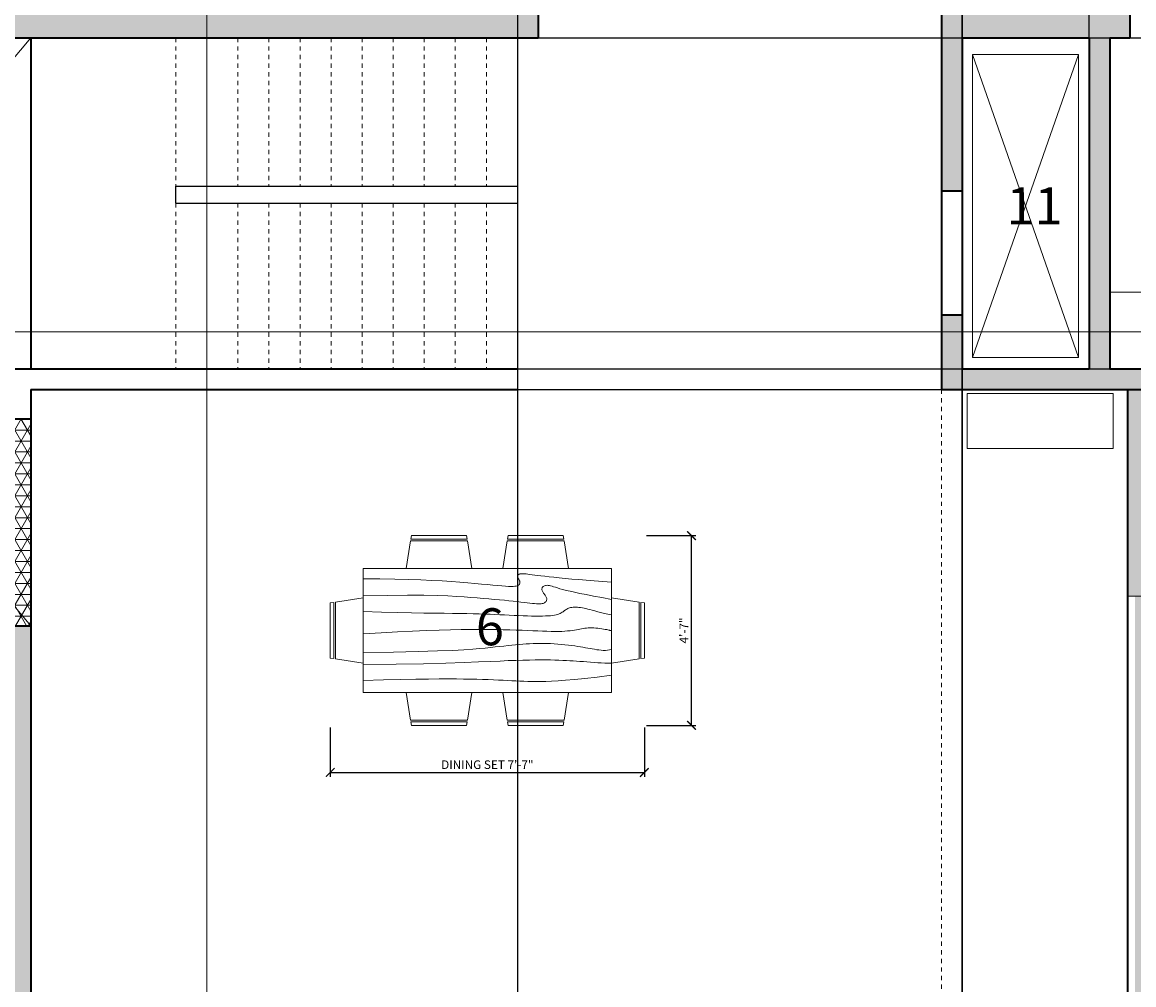
# Model space of a CAD drawing. Units: inches. Extents: x 3122 to 5933, y 1474 to 2995.
# Tile 7 of 12: x 5215 to 5538, y 2360 to 2639. Entities that reach past the tile are written whole.
import ezdxf

# ---------------------------------------------------------------- set-up
doc = ezdxf.new("R2010")
doc.units = ezdxf.units.IN
doc.linetypes.add('JIS_02_1.2', pattern=[2.5, 1.25, -1.25])
for name, color, linetype, lineweight in [('A-ANNO-DIMS', 2, 'Continuous', 18), ('A-ANNO-SYMB', 6, 'Continuous', 18), ('A-AREA-IDEN', 7, 'Continuous', 20), ('A-EQPM', 9, 'Continuous', 20), ('A-FLOR-FIXT', 9, 'Continuous', 18), ('A-FLOR-OPEN', 8, 'Continuous', 13), ('A-FLOR-OVHD', 8, 'JIS_02_1.2', 18), ('A-FLOR-STRS', 7, 'Continuous', 25), ('A-FLOR-STRS-OVHD', 8, 'JIS_02_1.2', 18), ('A-FURN', 8, 'Continuous', 18), ('A-GLAZ', 4, 'Continuous', 18), ('A-WALL', 7, 'Continuous', 35), ('A-WALL-PATT', 7, 'Continuous', 13), ('L-PLNT-PATT', 94, 'Continuous', 13)]:
    doc.layers.add(name, color=color, linetype=linetype, lineweight=lineweight)
doc.styles.get("Standard").update_dxf_attribs({"font": 'arial.ttf'})
doc.dimstyles.new('ISO-25', dxfattribs={"dimtxt": 2.5, "dimasz": 2.5, "dimexe": 1.25, "dimexo": 0.625, "dimtad": 1, "dimdec": 0, "dimlunit": 3, "dimtxsty": 'Standard', "dimblk": 'ARCHTICK', "dimcen": 2.5, "dimadec": 0, "dimazin": 0, "dimtfac": 1, "dimtdec": 0, "dimtmove": 0, "dimatfit": 3, "dimfxl": 1, "dimarcsym": 0})

# ---------------------------------------------------------------- blocks, each defined once
blk = doc.blocks.new('Dining Set - 36 x 72 in.')
for p, q in [((-22.2343, 26.00059), (-23.4847, 17.99762)), ((-22.2304, 26), (-5.7608, 26)), ((-22, 27.5), (-22.1562, 26.50042)), ((-5.8416, 26.5), (-22.1534, 26.5)), ((-22, 27.5), (-6, 27.5)), ((-5.8437, 26.49966), (-6, 27.5)), ((-4.5152, 17.99762), (-5.7655, 25.99926)), ((5.7657, 26.00059), (4.5153, 17.99762)), ((5.7696, 26), (22.2392, 26)), ((6, 27.5), (5.8438, 26.50042)), ((22.1584, 26.5), (5.8466, 26.5)), ((6, 27.5), (22, 27.5)), ((22.1563, 26.49966), (22, 27.5)), ((23.4848, 17.99762), (22.2345, 25.99926)), ((36, 18), (-36, 18)), ((-36, 18), (-36, -18)), ((36, -18), (36, 18)), ((-45.5, 8), (-44.5004, 8.15617)), ((-45.5, 8), (-45.5, -8)), ((-44.5, -8.15843), (-44.5, 8.15338)), ((-44.0006, 8.23428), (-35.9976, 9.48474)), ((-44, 8.23041), (-44, -8.23915)), ((44.0006, 8.23428), (35.9976, 9.48474)), ((44, 8.23041), (44, -8.23915)), ((44.5, -8.15843), (44.5, 8.15338)), ((45.5, 8), (44.5005, 8.15617)), ((45.5, 8), (45.5, -8)), ((-44.4997, -8.15631), (-45.5, -8)), ((-35.9976, -9.48476), (-43.9993, -8.2345)), ((35.9976, -9.48476), (43.9993, -8.2345)), ((44.4997, -8.15631), (45.5, -8)), ((-36, -18), (36, -18)), ((-22.2343, -26.0006), (-23.4847, -17.99762)), ((-4.5152, -17.99762), (-5.7655, -25.99928)), ((5.7657, -26.0006), (4.5153, -17.99762)), ((23.4848, -17.99762), (22.2345, -25.99928)), ((-22.2304, -26), (-5.7608, -26)), ((-22, -27.5), (-22.1562, -26.50044)), ((-5.8416, -26.5), (-22.1534, -26.5)), ((-22, -27.5), (-6, -27.5)), ((-5.8437, -26.49967), (-6, -27.5)), ((5.7696, -26), (22.2392, -26)), ((6, -27.5), (5.8438, -26.50044)), ((22.1584, -26.5), (5.8466, -26.5)), ((6, -27.5), (22, -27.5)), ((22.1563, -26.49967), (22, -27.5))]:
    blk.add_line(p, q)
for points in [[(-36, 15), (-31.1772, 14.97754), (-26.8079, 14.91406), (-22.8538, 14.81543), (-19.276, 14.6875), (-16.0362, 14.53613), (-13.0957, 14.36718), (-10.4159, 14.18652), (-7.9583, 14), (-5.6904, 13.81315), (-3.6035, 13.63021), (-1.6954, 13.45508), (0.0365, 13.29166), (1.5945, 13.14388), (2.9811, 13.01562), (4.1988, 12.9108), (5.25, 12.83333), (6.1393, 12.78613), (6.8802, 12.76823), (7.4883, 12.77767), (7.9792, 12.8125), (8.3685, 12.87077), (8.6719, 12.95052), (8.9049, 13.0498), (9.0833, 13.16666), (9.2205, 13.29899), (9.3216, 13.44401), (9.3895, 13.59879), (9.4271, 13.76041), (9.4373, 13.92594), (9.4232, 14.09245), (9.3875, 14.257), (9.3333, 14.41666), (9.2638, 14.56917), (9.1836, 14.71484), (9.0975, 14.85465), (9.0104, 14.98958), (8.9272, 15.1206), (8.8529, 15.2487), (8.7922, 15.37483), (8.75, 15.5), (8.7305, 15.62467), (8.7344, 15.74739), (8.7617, 15.86621), (8.8125, 15.97916), (8.8867, 16.08431), (8.9844, 16.17968), (9.1055, 16.26334), (9.25, 16.33333), (9.4189, 16.38802), (9.6172, 16.42708), (9.8506, 16.45052), (10.125, 16.45833), (10.4463, 16.45052), (10.8203, 16.42708), (11.2529, 16.38802), (11.75, 16.33333), (12.3184, 16.26318), (12.9694, 16.17838), (13.7151, 16.07991), (14.5677, 15.96875), (15.5395, 15.84586), (16.6426, 15.71224), (17.8893, 15.56884), (19.2917, 15.41666), (20.859, 15.25667), (22.5879, 15.08984), (24.4721, 14.91715), (26.5052, 14.73958), (28.6809, 14.5581), (30.9929, 14.3737), (33.4347, 14.18733), (36, 14)], [(-36, 10), (-28.9766, 10.14274), (-23.1725, 10.20442), (-18.4241, 10.19775), (-14.5677, 10.13541), (-11.4399, 10.03011), (-8.877, 9.89453), (-6.7154, 9.74137), (-4.7917, 9.58333), (-2.9698, 9.43082), (-1.2246, 9.28515), (0.4415, 9.14534), (2.026, 9.01041), (3.5266, 8.87939), (4.9408, 8.7513), (6.266, 8.62516), (7.5, 8.5), (8.6411, 8.37549), (9.6914, 8.2539), (10.6538, 8.13818), (11.5312, 8.03125), (12.3267, 7.93603), (13.043, 7.85547), (13.6831, 7.79248), (14.25, 7.75), (14.7471, 7.7303), (15.1797, 7.73307), (15.5537, 7.75732), (15.875, 7.80208), (16.1494, 7.86637), (16.3828, 7.94922), (16.5811, 8.04964), (16.75, 8.16666), (16.8944, 8.29915), (17.0143, 8.44531), (17.1089, 8.60319), (17.1771, 8.77083), (17.218, 8.94629), (17.2305, 9.1276), (17.2137, 9.31282), (17.1667, 9.5), (17.0895, 9.6875), (16.987, 9.875), (16.8649, 10.0625), (16.7292, 10.25), (16.5856, 10.4375), (16.4401, 10.625), (16.2985, 10.8125), (16.1667, 11), (16.05, 11.18733), (15.9518, 11.3737), (15.8752, 11.5581), (15.8229, 11.73958), (15.798, 11.91715), (15.8034, 12.08984), (15.842, 12.25667), (15.9167, 12.41666), (16.0295, 12.56836), (16.1784, 12.70833), (16.3605, 12.83268), (16.5729, 12.9375), (16.8127, 13.01888), (17.0768, 13.07291), (17.3625, 13.0957), (17.6667, 13.08333), (17.9894, 13.03312), (18.3418, 12.94726), (18.7382, 12.82918), (19.1927, 12.68229), (19.7195, 12.51001), (20.3327, 12.31575), (21.0465, 12.10294), (21.875, 11.875), (22.8357, 11.63354), (23.959, 11.37304), (25.2786, 11.08618), (26.8282, 10.76562), (28.6414, 10.40405), (30.752, 9.99414), (33.1936, 9.52856), (36, 9)], [(-36, 5.5), (-30.7157, 5.3348), (-26.069, 5.20963), (-21.9946, 5.11767), (-18.4271, 5.05208), (-15.3009, 5.00602), (-12.5508, 4.97265), (-10.1112, 4.94515), (-7.9167, 4.91666), (-5.909, 4.88167), (-4.0586, 4.83984), (-2.3429, 4.79215), (-0.7396, 4.73958), (0.7739, 4.6831), (2.22, 4.6237), (3.6213, 4.56233), (5, 4.5), (6.373, 4.43782), (7.7344, 4.3776), (9.0723, 4.32129), (10.375, 4.27083), (11.6309, 4.22819), (12.8281, 4.19531), (13.9551, 4.17415), (15, 4.16666), (15.954, 4.17448), (16.819, 4.19791), (17.6001, 4.23698), (18.3021, 4.29166), (18.9299, 4.36198), (19.4883, 4.44791), (19.9823, 4.54948), (20.4167, 4.66666), (20.7969, 4.79899), (21.1302, 4.94401), (21.4245, 5.09879), (21.6875, 5.26041), (21.9271, 5.42594), (22.1511, 5.59245), (22.3672, 5.757), (22.5834, 5.91666), (22.8065, 6.06868), (23.0404, 6.21093), (23.2879, 6.34147), (23.5521, 6.45833), (23.8358, 6.55957), (24.142, 6.64323), (24.4735, 6.70735), (24.8334, 6.75), (25.2235, 6.76969), (25.642, 6.76692), (26.0858, 6.74267), (26.5521, 6.69791), (27.0379, 6.63362), (27.5404, 6.55078), (28.0565, 6.45036), (28.5834, 6.33333), (29.1242, 6.19987), (29.7071, 6.04687), (30.3661, 5.87044), (31.1354, 5.66666), (32.0493, 5.43164), (33.142, 5.16146), (34.4475, 4.85221), (36, 4.5)], [(-36, -1), (-30.7915, -0.6591), (-26.0195, -0.38216), (-21.6519, -0.16284), (-17.6563, 0.00521), (-14.0005, 0.12833), (-10.6523, 0.21289), (-7.5796, 0.26522), (-4.75, 0.29166), (-2.134, 0.29793), (0.2878, 0.28711), (2.5317, 0.26163), (4.6146, 0.22396), (6.5529, 0.17651), (8.3633, 0.12174), (10.0623, 0.06209), (11.6667, 0), (13.1899, -0.06201), (14.6341, -0.1211), (15.9982, -0.17432), (17.2813, -0.21875), (18.4823, -0.25147), (19.6003, -0.26953), (20.6343, -0.27002), (21.5834, -0.25), (22.4481, -0.20768), (23.2357, -0.14584), (23.9549, -0.06836), (24.6146, 0.02083), (25.2235, 0.11784), (25.7904, 0.21875), (26.3241, 0.31966), (26.8334, 0.41666), (27.3265, 0.50618), (27.8099, 0.58593), (28.2894, 0.65397), (28.7709, 0.70833), (29.2601, 0.74707), (29.763, 0.76823), (30.2855, 0.76985), (30.8334, 0.75), (31.4088, 0.70784), (31.9994, 0.64713), (32.589, 0.57275), (33.1615, 0.48958), (33.7008, 0.4025), (34.1908, 0.3164), (34.6153, 0.23616), (34.9584, 0.16666), (35.2099, 0.11165), (35.3848, 0.07031), (35.504, 0.04069), (35.5886, 0.02083), (35.6594, 0.00879), (35.7377, 0.0026), (35.8442, 0.00032), (36, 0)], [(-36, -6.5), (-27.1843, -6.31267), (-20.084, -6.1263), (-14.469, -5.9419), (-10.1094, -5.76042), (-6.7752, -5.58285), (-4.2363, -5.41016), (-2.2629, -5.24333), (-0.625, -5.08334), (0.8708, -4.93099), (2.2715, -4.78646), (3.5872, -4.64974), (4.8281, -4.52084), (6.0046, -4.39974), (7.127, -4.28646), (8.2053, -4.18099), (9.25, -4.08334), (10.2705, -3.99382), (11.2734, -3.91407), (12.2647, -3.84603), (13.25, -3.79167), (14.2354, -3.75293), (15.2266, -3.73177), (16.2295, -3.73015), (17.25, -3.75), (18.2912, -3.79248), (19.3451, -3.85547), (20.4009, -3.93604), (21.4479, -4.03125), (22.4754, -4.13819), (23.4727, -4.25391), (24.4289, -4.37549), (25.3334, -4.5), (26.1785, -4.62492), (26.9694, -4.74935), (27.7145, -4.87281), (28.4219, -4.99479), (29.1, -5.11483), (29.7572, -5.23242), (30.4016, -5.34709), (31.0417, -5.45834), (31.6837, -5.56437), (32.3262, -5.65821), (32.9658, -5.73153), (33.599, -5.77604), (34.2224, -5.78345), (34.8327, -5.74545), (35.4264, -5.65373), (36, -5.5)], [(-36, -10), (-26.4022, -9.81299), (-18.4675, -9.62891), (-11.9839, -9.45069), (-6.7396, -9.28125), (-2.5226, -9.12354), (0.8789, -8.98047), (3.6769, -8.85498), (6.0833, -8.75), (8.2767, -8.66765), (10.3021, -8.60677), (12.1712, -8.56543), (13.8958, -8.54167), (15.4876, -8.53353), (16.9583, -8.53907), (18.3197, -8.55632), (19.5834, -8.58334), (20.7616, -8.61841), (21.8685, -8.66081), (22.9188, -8.71004), (23.9271, -8.76563), (24.9081, -8.82707), (25.8763, -8.89388), (26.8465, -8.96558), (27.8334, -9.04167), (28.8474, -9.12118), (29.8828, -9.20117), (30.93, -9.27824), (31.9792, -9.34896), (33.0205, -9.40991), (34.0443, -9.45768), (35.0407, -9.48885), (36, -9.5)], [(-36, -14.5), (-30.0881, -14.33513), (-25.0332, -14.21224), (-20.7312, -14.12647), (-17.0781, -14.07292), (-13.97, -14.04671), (-11.3027, -14.04297), (-8.9724, -14.05681), (-6.875, -14.08334), (-4.9224, -14.11833), (-3.0905, -14.16016), (-1.3709, -14.20785), (0.2448, -14.26042), (1.7647, -14.3169), (3.1973, -14.3763), (4.5507, -14.43767), (5.8333, -14.5), (7.0554, -14.5621), (8.235, -14.62175), (9.3922, -14.67652), (10.5469, -14.72396), (11.7192, -14.76164), (12.929, -14.78711), (14.1965, -14.79794), (15.5417, -14.79167), (16.9933, -14.76424), (18.6152, -14.70508), (20.4804, -14.60197), (22.6615, -14.44271), (25.2312, -14.21509), (28.2624, -13.9069), (31.8277, -13.50594), (36, -13)]]:
    blk.add_lwpolyline(points)
blk = doc.blocks.new('_ArchTick')
at = {"color": 0, "linetype": 'ByBlock', "const_width": 0.15}
blk.add_lwpolyline([(-0.5, -0.5), (0.5, 0.5)], dxfattribs=at)
blk = doc.blocks.new('*D82')
at = {"layer": 'A-ANNO-DIMS', "color": 0, "lineweight": -2, "transparency": 16777216}
for p, q in [((5304.74, 2434.72), (5304.74, 2420.45)), ((5395.74, 2434.72), (5395.74, 2420.45)), ((5304.74, 2421.7), (5395.74, 2421.7))]:
    blk.add_line(p, q, dxfattribs=at)
at = {"layer": 'Defpoints', "color": 0, "transparency": 16777216}
for p in [(5304.74, 2435.35), (5395.74, 2435.35), (5395.74, 2421.7)]:
    blk.add_point(p, dxfattribs=at)
at = {"layer": 'A-ANNO-DIMS', "color": 0, "lineweight": -2, "transparency": 16777216, "xscale": 2.5, "yscale": 2.5, "zscale": 2.5, "rotation": 180}
blk.add_blockref('_ArchTick', (5304.74, 2421.7), dxfattribs=at)
at = {"layer": 'A-ANNO-DIMS', "color": 0, "lineweight": -2, "transparency": 16777216, "xscale": 2.5, "yscale": 2.5, "zscale": 2.5}
blk.add_blockref('_ArchTick', (5395.74, 2421.7), dxfattribs=at)
at = {"layer": 'A-ANNO-DIMS', "color": 0, "transparency": 16777216, "insert": (5350.24, 2423.62), "char_height": 2.5, "attachment_point": 5}
blk.add_mtext('DINING SET 7\'-7"', dxfattribs=at)
blk = doc.blocks.new('*D83')
at = {"layer": 'A-ANNO-DIMS', "color": 0, "lineweight": -2, "transparency": 16777216}
for p, q in [((5396.36, 2490.35), (5410.64, 2490.35)), ((5409.39, 2435.35), (5409.39, 2490.35)), ((5396.36, 2435.35), (5410.64, 2435.35))]:
    blk.add_line(p, q, dxfattribs=at)
at = {"layer": 'Defpoints', "color": 0, "transparency": 16777216}
for p in [(5395.74, 2490.35), (5409.39, 2490.35), (5395.74, 2435.35)]:
    blk.add_point(p, dxfattribs=at)
at = {"layer": 'A-ANNO-DIMS', "color": 0, "lineweight": -2, "transparency": 16777216, "xscale": 2.5, "yscale": 2.5, "zscale": 2.5}
for p, rotation in [((5409.39, 2490.35), 90), ((5409.39, 2435.35), 270)]:
    blk.add_blockref('_ArchTick', p, dxfattribs=dict(at, rotation=rotation))
at = {"layer": 'A-ANNO-DIMS', "color": 0, "transparency": 16777216, "insert": (5407.51, 2462.85), "char_height": 2.5, "attachment_point": 5, "rotation": 90}
blk.add_mtext('4\'-7"', dxfattribs=at)
blk = doc.blocks.new('*D94')
at = {"layer": 'A-ANNO-DIMS', "color": 0, "lineweight": -2, "transparency": 16777216}
for p, q in [((5064.96, 1916.52), (5064.96, 2990.75)), ((5064.96, 2989.5), (5487.87, 2989.5)), ((5487.87, 1916.52), (5487.87, 2990.75))]:
    blk.add_line(p, q, dxfattribs=at)
at = {"layer": 'Defpoints', "color": 0, "transparency": 16777216}
for p in [(5487.87, 2989.5), (5064.96, 1915.9), (5487.87, 1915.9)]:
    blk.add_point(p, dxfattribs=at)
at = {"layer": 'A-ANNO-DIMS', "color": 0, "lineweight": -2, "transparency": 16777216, "xscale": 2.5, "yscale": 2.5, "zscale": 2.5, "rotation": 180}
blk.add_blockref('_ArchTick', (5064.96, 2989.5), dxfattribs=at)
at = {"layer": 'A-ANNO-DIMS', "color": 0, "lineweight": -2, "transparency": 16777216, "xscale": 2.5, "yscale": 2.5, "zscale": 2.5}
blk.add_blockref('_ArchTick', (5487.87, 2989.5), dxfattribs=at)
at = {"layer": 'A-ANNO-DIMS', "color": 0, "transparency": 16777216, "insert": (5276.42, 2991.41), "char_height": 2.5, "attachment_point": 5}
blk.add_mtext('35\'-3"', dxfattribs=at)
blk = doc.blocks.new('*D108')
at = {"layer": 'A-ANNO-DIMS', "color": 0, "lineweight": -2, "transparency": 16777216}
for p, q in [((5178.96, 2643.06), (5178.96, 1792.93)), ((5358.96, 2643.06), (5358.96, 1792.93)), ((5178.96, 1794.18), (5358.96, 1794.18))]:
    blk.add_line(p, q, dxfattribs=at)
at = {"layer": 'Defpoints', "color": 0, "transparency": 16777216}
for p in [(5178.96, 2643.69), (5358.96, 2643.69), (5358.96, 1794.18)]:
    blk.add_point(p, dxfattribs=at)
at = {"layer": 'A-ANNO-DIMS', "color": 0, "lineweight": -2, "transparency": 16777216, "xscale": 2.5, "yscale": 2.5, "zscale": 2.5, "rotation": 180}
blk.add_blockref('_ArchTick', (5178.96, 1794.18), dxfattribs=at)
at = {"layer": 'A-ANNO-DIMS', "color": 0, "lineweight": -2, "transparency": 16777216, "xscale": 2.5, "yscale": 2.5, "zscale": 2.5}
blk.add_blockref('_ArchTick', (5358.96, 1794.18), dxfattribs=at)
at = {"layer": 'A-ANNO-DIMS', "color": 0, "transparency": 16777216, "insert": (5268.96, 1796.08), "char_height": 2.5, "attachment_point": 5}
blk.add_mtext('15\'-0"', dxfattribs=at)
blk = doc.blocks.new('*D110')
at = {"layer": 'A-ANNO-DIMS', "color": 0, "lineweight": -2, "transparency": 16777216}
for p, q in [((5487.87, 2643.06), (5487.87, 1792.93)), ((5670.96, 2643.06), (5670.96, 1792.93)), ((5487.87, 1794.18), (5670.96, 1794.18))]:
    blk.add_line(p, q, dxfattribs=at)
at = {"layer": 'Defpoints', "color": 0, "transparency": 16777216}
for p in [(5487.87, 2643.69), (5670.96, 2643.69), (5670.96, 1794.18)]:
    blk.add_point(p, dxfattribs=at)
at = {"layer": 'A-ANNO-DIMS', "color": 0, "lineweight": -2, "transparency": 16777216, "xscale": 2.5, "yscale": 2.5, "zscale": 2.5, "rotation": 180}
blk.add_blockref('_ArchTick', (5487.87, 1794.18), dxfattribs=at)
at = {"layer": 'A-ANNO-DIMS', "color": 0, "lineweight": -2, "transparency": 16777216, "xscale": 2.5, "yscale": 2.5, "zscale": 2.5}
blk.add_blockref('_ArchTick', (5670.96, 1794.18), dxfattribs=at)
at = {"layer": 'A-ANNO-DIMS', "color": 0, "transparency": 16777216, "insert": (5579.42, 1796.09), "char_height": 2.5, "attachment_point": 5}
blk.add_mtext('15\'-3"', dxfattribs=at)
blk = doc.blocks.new('*D113')
at = {"layer": 'A-ANNO-DIMS', "color": 0, "lineweight": -2, "transparency": 16777216}
for p, q in [((5218.59, 2634.69), (5931.98, 2634.69)), ((5930.73, 2538.69), (5930.73, 2634.69)), ((5218.59, 2538.69), (5931.98, 2538.69))]:
    blk.add_line(p, q, dxfattribs=at)
at = {"layer": 'Defpoints', "color": 0, "transparency": 16777216}
for p in [(5217.96, 2634.69), (5930.73, 2634.69), (5217.96, 2538.69)]:
    blk.add_point(p, dxfattribs=at)
at = {"layer": 'A-ANNO-DIMS', "color": 0, "lineweight": -2, "transparency": 16777216, "xscale": 2.5, "yscale": 2.5, "zscale": 2.5}
for p, rotation in [((5930.73, 2634.69), 90), ((5930.73, 2538.69), 270)]:
    blk.add_blockref('_ArchTick', p, dxfattribs=dict(at, rotation=rotation))
at = {"layer": 'A-ANNO-DIMS', "color": 0, "transparency": 16777216, "insert": (5928.83, 2586.69), "char_height": 2.5, "attachment_point": 5, "rotation": 90}
blk.add_mtext('8\'-0"', dxfattribs=at)
blk = doc.blocks.new('*D114')
at = {"layer": 'A-ANNO-DIMS', "color": 0, "lineweight": -2, "transparency": 16777216}
for p, q in [((5487.87, 2539.31), (5487.87, 2990.75)), ((5487.87, 2989.5), (5524.65, 2989.5)), ((5524.65, 2539.31), (5524.65, 2990.75))]:
    blk.add_line(p, q, dxfattribs=at)
at = {"layer": 'Defpoints', "color": 0, "transparency": 16777216}
for p in [(5524.65, 2989.5), (5487.87, 2538.69), (5524.65, 2538.69)]:
    blk.add_point(p, dxfattribs=at)
at = {"layer": 'A-ANNO-DIMS', "color": 0, "lineweight": -2, "transparency": 16777216, "xscale": 2.5, "yscale": 2.5, "zscale": 2.5, "rotation": 180}
blk.add_blockref('_ArchTick', (5487.87, 2989.5), dxfattribs=at)
at = {"layer": 'A-ANNO-DIMS', "color": 0, "lineweight": -2, "transparency": 16777216, "xscale": 2.5, "yscale": 2.5, "zscale": 2.5}
blk.add_blockref('_ArchTick', (5524.65, 2989.5), dxfattribs=at)
at = {"layer": 'A-ANNO-DIMS', "color": 0, "transparency": 16777216, "insert": (5506.26, 2991.41), "char_height": 2.5, "attachment_point": 5}
blk.add_mtext('3\'-1"', dxfattribs=at)
blk = doc.blocks.new('*D115')
at = {"layer": 'A-ANNO-DIMS', "color": 0, "lineweight": -2, "transparency": 16777216}
for p, q in [((5217.96, 2532.06), (5217.96, 1792.93)), ((5535.87, 2532.06), (5535.87, 1792.93)), ((5217.96, 1794.18), (5535.87, 1794.18))]:
    blk.add_line(p, q, dxfattribs=at)
at = {"layer": 'Defpoints', "color": 0, "transparency": 16777216}
for p in [(5217.96, 2532.69), (5535.87, 2532.69), (5535.87, 1794.18)]:
    blk.add_point(p, dxfattribs=at)
at = {"layer": 'A-ANNO-DIMS', "color": 0, "lineweight": -2, "transparency": 16777216, "xscale": 2.5, "yscale": 2.5, "zscale": 2.5, "rotation": 180}
blk.add_blockref('_ArchTick', (5217.96, 1794.18), dxfattribs=at)
at = {"layer": 'A-ANNO-DIMS', "color": 0, "lineweight": -2, "transparency": 16777216, "xscale": 2.5, "yscale": 2.5, "zscale": 2.5}
blk.add_blockref('_ArchTick', (5535.87, 1794.18), dxfattribs=at)
at = {"layer": 'A-ANNO-DIMS', "color": 0, "transparency": 16777216, "insert": (5376.92, 1796.08), "char_height": 2.5, "attachment_point": 5}
blk.add_mtext('26\'-6"', dxfattribs=at)
blk = doc.blocks.new('*D116')
at = {"layer": 'A-ANNO-DIMS', "color": 0, "lineweight": -2, "transparency": 16777216}
for p, q in [((5218.59, 2532.69), (5931.98, 2532.69)), ((5930.73, 2352.69), (5930.73, 2532.69)), ((5218.59, 2352.69), (5931.98, 2352.69))]:
    blk.add_line(p, q, dxfattribs=at)
at = {"layer": 'Defpoints', "color": 0, "transparency": 16777216}
for p in [(5217.96, 2532.69), (5930.73, 2532.69), (5217.96, 2352.69)]:
    blk.add_point(p, dxfattribs=at)
at = {"layer": 'A-ANNO-DIMS', "color": 0, "lineweight": -2, "transparency": 16777216, "xscale": 2.5, "yscale": 2.5, "zscale": 2.5}
for p, rotation in [((5930.73, 2532.69), 90), ((5930.73, 2352.69), 270)]:
    blk.add_blockref('_ArchTick', p, dxfattribs=dict(at, rotation=rotation))
at = {"layer": 'A-ANNO-DIMS', "color": 0, "transparency": 16777216, "insert": (5928.83, 2442.69), "char_height": 2.5, "attachment_point": 5, "rotation": 90}
blk.add_mtext('15\'-0"', dxfattribs=at)

msp = doc.modelspace()

# ---------------------------------------------------------------- hatches: boundary and pattern name
at = {"layer": 'A-WALL-PATT'}
h = msp.add_hatch(color=256, dxfattribs=at)
h.dxf.hatch_style = 1
h.paths.add_polyline_path([(5073.96, 2454.69), (5101.59, 2454.69), (5101.59, 2459.69), (5101.59, 2463.69), (5073.96, 2463.69), (5073.96, 2634.69), (5169.96, 2634.69), (5364.96, 2634.69), (5364.96, 2643.69), (5364.96, 2667.06), (5358.96, 2667.06), (5358.96, 2643.69), (5178.96, 2643.69), (5178.96, 2655.69), (5169.96, 2655.69), (5169.96, 2643.69), (5073.96, 2643.69), (5073.96, 2745.9), (5124.13, 2745.9), (5124.13, 2754.9), (5073.96, 2754.9), (5073.96, 2866.9), (5169.96, 2866.9), (5169.96, 2818.9), (5169.96, 2812.9), (5169.96, 2754.9), (5154.13, 2754.9), (5154.13, 2745.9), (5169.96, 2745.9), (5169.96, 2691.69), (5178.96, 2691.69), (5178.96, 2812.9), (5178.96, 2818.9), (5178.96, 2875.9), (5064.96, 2875.9), (5064.96, 2055.71), (5217.96, 2055.71), (5217.96, 2464.19), (5212.96, 2464.19), (5212.96, 2463.69), (5148.19, 2463.69), (5148.19, 2459.69), (5148.19, 2454.69), (5158.96, 2454.69), (5158.96, 2450.72), (5156.04, 2450.72), (5156.04, 2447.72), (5158.96, 2447.72), (5158.96, 2425.1), (5164.96, 2425.1), (5164.96, 2447.72), (5167.71, 2447.72), (5167.71, 2450.72), (5164.96, 2450.72), (5164.96, 2454.69), (5212.96, 2454.69), (5212.96, 2064.71), (5073.96, 2064.71), (5073.96, 2322.69), (5158.96, 2322.69), (5164.96, 2322.69), (5164.96, 2328.69), (5158.96, 2328.69), (5073.96, 2328.69)])
h = msp.add_hatch(color=256, dxfattribs=at)
h.dxf.hatch_style = 1
h.paths.add_polyline_path([(5536.42, 2643.69), (5487.87, 2643.69), (5487.87, 2667.06), (5485.81, 2667.06), (5481.87, 2667.06), (5481.87, 2643.69), (5481.87, 2590.35), (5487.87, 2590.35), (5487.87, 2634.69), (5524.65, 2634.69), (5524.65, 2538.69), (5487.87, 2538.69), (5487.87, 2554.35), (5481.87, 2554.35), (5481.87, 2532.69), (5524.65, 2532.69), (5658.65, 2532.69), (5718.65, 2532.69), (5718.65, 2501.93), (5724.65, 2501.93), (5724.65, 2549.4), (5718.65, 2549.4), (5718.65, 2538.69), (5658.65, 2538.69), (5658.65, 2573.57), (5658.59, 2573.63), (5654.65, 2573.63), (5654.65, 2538.69), (5594.65, 2538.69), (5594.65, 2573.57), (5594.59, 2573.63), (5590.65, 2573.63), (5590.65, 2538.69), (5530.65, 2538.69), (5530.65, 2634.69), (5536.42, 2634.69)])
h.paths.add_polyline_path([(5735.69, 2643.69), (5679.96, 2643.69), (5679.96, 2710.77), (5720.44, 2710.77), (5720.44, 2687.32), (5737.79, 2687.32), (5737.79, 2692.32), (5725.44, 2692.32), (5725.44, 2715.77), (5679.96, 2715.77), (5679.96, 2866.9), (5775.96, 2866.9), (5775.96, 2692.32), (5773.79, 2692.32), (5773.79, 2687.32), (5775.96, 2687.32), (5775.96, 2643.69), (5775.96, 2591.85), (5784.96, 2591.85), (5784.96, 2875.9), (5670.96, 2875.9), (5670.96, 2818.9), (5412.4, 2818.9), (5412.4, 2812.9), (5460.96, 2812.9), (5460.96, 2719.12), (5404.54, 2719.12), (5404.54, 2713.12), (5466.96, 2713.12), (5481.87, 2713.12), (5481.87, 2703.06), (5487.87, 2703.06), (5487.87, 2719.12), (5466.96, 2719.12), (5466.96, 2812.9), (5670.96, 2812.9), (5670.96, 2643.69), (5572.42, 2643.69), (5572.42, 2634.69), (5718.65, 2634.69), (5718.65, 2549.4), (5724.65, 2549.4), (5724.65, 2591.85), (5739.96, 2591.85), (5739.96, 2596.85), (5724.65, 2596.85), (5724.65, 2634.69), (5735.69, 2634.69)])
h.paths.add_polyline_path([(5594.65, 2634.69), (5590.65, 2634.69), (5590.65, 2603.63), (5594.65, 2603.63)], flags=17)
h.paths.add_polyline_path([(5724.65, 2441.93), (5718.65, 2441.93), (5718.65, 2336.51), (5724.65, 2336.51)])
h.paths.add_polyline_path([(5724.65, 2276.51), (5718.65, 2276.51), (5718.65, 2250.49), (5713.26, 2250.49), (5713.26, 2244.39), (5724.65, 2244.39)])
h.paths.add_polyline_path([(5689.26, 2250.49), (5540.87, 2250.49), (5540.87, 2317.46), (5535.87, 2317.46), (5535.87, 2244.39), (5689.26, 2244.39)])
h.paths.add_polyline_path([(5540.87, 2532.69), (5535.87, 2532.69), (5535.87, 2472.78), (5540.87, 2472.78)])
h.paths.add_polyline_path([(5540.87, 2472.78), (5537.87, 2472.78), (5537.87, 2346.69), (5537.87, 2317.46), (5540.87, 2317.46)])
at = {"layer": 'L-PLNT-PATT'}
h = msp.add_hatch(dxfattribs=at)
h.set_pattern_fill('NET3', color=256)
h.paths.add_polyline_path([(5217.96, 2524.19), (5212.96, 2524.19), (5212.96, 2532.69), (5197.46, 2532.69), (5197.46, 2634.69), (5169.96, 2634.69), (5101.59, 2634.69), (5101.59, 2463.69), (5101.59, 2459.69), (5148.19, 2459.69), (5148.19, 2463.69), (5212.96, 2463.69), (5212.96, 2464.19), (5217.96, 2464.19)])
h.paths.add_polyline_path([(5125.86, 2509.63), (5149.73, 2509.63), (5149.73, 2490.31), (5125.86, 2490.31)], flags=16)
h.paths.add_polyline_path([(5125.86, 2523.69), (5125.86, 2579.54), (5149.73, 2579.54), (5149.73, 2523.69)], flags=16)
h.paths.add_polyline_path([(5172.93, 2505.39, -0.929737), (5184.73, 2504.53, -0.91381), (5172.96, 2503.47, -0.960136), (5153.44, 2504.26, -0.943722)], flags=16)
h.paths.add_polyline_path([(5150.78, 2528.95, -1), (5168.14, 2528.95, -1)], flags=16)
h.paths.add_polyline_path([(5150.99, 2552.62, -1), (5171.14, 2552.62, -1)], flags=16)
h.paths.add_polyline_path([(5169.25, 2521.97, -1), (5181.9, 2521.97, -1)], flags=16)
h.paths.add_polyline_path([(5171.47, 2540.81, -1), (5186.66, 2540.81, -1)], flags=16)
h.paths.add_polyline_path([(5182.81, 2513.65, -1), (5196.27, 2513.65, -1)], flags=16)
h.paths.add_polyline_path([(5154.93, 2577.08, -1), (5176.33, 2577.08, -1)], flags=16)
h.paths.add_polyline_path([(5172.55, 2564.2, -1), (5180.74, 2564.2, -1)], flags=16)
h.paths.add_polyline_path([(5178.29, 2572.78, -1), (5187.9, 2572.78, -1)], flags=16)
h.paths.add_polyline_path([(5125.86, 2595.84), (5125.86, 2615.17), (5149.73, 2615.17), (5149.73, 2595.84)], flags=16)
h.paths.add_polyline_path([(5169.27, 2597.2, -1), (5179.18, 2597.2, -1)], flags=16)
h.paths.add_polyline_path([(5159.45, 2603.11, -1), (5170.74, 2603.11, -1)], flags=16)
h.paths.add_polyline_path([(5166.7, 2616.79, -1), (5186.05, 2616.79, -1)], flags=16)
h.paths.add_polyline_path([(5129.27, 2547.83), (5151.41, 2547.84), (5151.4, 2564.27), (5129.26, 2564.26)], flags=24)

# ---------------------------------------------------------------- linework, layer by layer
at = {"layer": 'A-ANNO-SYMB'}
for p, q in [((5268.96, 2933.31), (5268.96, 1850.37)), ((5874.48, 2549.4), (4977.78, 2549.4))]:
    msp.add_line(p, q, dxfattribs=at)
at = {"layer": 'A-EQPM'}
for p, q in [((5490.8, 2629.85), (5521.5, 2541.94)), ((5490.8, 2541.94), (5521.5, 2629.85))]:
    msp.add_line(p, q, dxfattribs=at)
msp.add_lwpolyline([(5490.8, 2629.85), (5521.5, 2629.85), (5521.5, 2541.94), (5490.8, 2541.94)], close=True, dxfattribs=at)
at = {"layer": 'A-FLOR-FIXT'}
msp.add_line((5590.65, 2560.9), (5530.65, 2560.9), dxfattribs=at)
at = {"layer": 'A-FLOR-OPEN'}
for p, q in [((5073.96, 2634.69), (5217.96, 2464.19)), ((5073.96, 2463.69), (5217.96, 2634.69))]:
    msp.add_line(p, q, dxfattribs=at)
at = {"layer": 'A-FLOR-OVHD'}
for p, q in [((5364.96, 2634.69), (5481.87, 2634.69)), ((5358.96, 2538.69), (5481.87, 2538.69)), ((5358.96, 2532.69), (5481.87, 2532.69)), ((5481.87, 2532.69), (5481.87, 2352.69)), ((5487.87, 2532.69), (5487.87, 2352.69))]:
    msp.add_line(p, q, dxfattribs=at)
at = {"layer": 'A-FLOR-STRS'}
for p, q in [((5259.96, 2591.69), (5358.96, 2591.69)), ((5259.96, 2586.69), (5259.96, 2591.69)), ((5259.96, 2586.69), (5358.96, 2586.69))]:
    msp.add_line(p, q, dxfattribs=at)
at = {"layer": 'A-FLOR-STRS-OVHD'}
for p, q in [((5259.96, 2634.69), (5259.96, 2591.69)), ((5268.96, 2634.69), (5268.96, 2591.69)), ((5277.96, 2634.69), (5277.96, 2591.69)), ((5286.96, 2634.69), (5286.96, 2591.69)), ((5295.96, 2634.69), (5295.96, 2591.69)), ((5304.96, 2634.69), (5304.96, 2591.69)), ((5313.96, 2634.69), (5313.96, 2591.69)), ((5322.96, 2634.69), (5322.96, 2591.69)), ((5331.96, 2634.69), (5331.96, 2591.69)), ((5340.96, 2634.69), (5340.96, 2591.69)), ((5349.96, 2634.69), (5349.96, 2591.69)), ((5358.96, 2634.69), (5358.96, 2591.69)), ((5259.96, 2586.69), (5259.96, 2538.69)), ((5268.96, 2586.69), (5268.96, 2538.69)), ((5277.96, 2586.69), (5277.96, 2538.69)), ((5286.96, 2586.69), (5286.96, 2538.69)), ((5295.96, 2586.69), (5295.96, 2538.69)), ((5304.96, 2586.69), (5304.96, 2538.69)), ((5313.96, 2586.69), (5313.96, 2538.69)), ((5322.96, 2586.69), (5322.96, 2538.69)), ((5331.96, 2586.69), (5331.96, 2538.69)), ((5340.96, 2586.69), (5340.96, 2538.69)), ((5349.96, 2586.69), (5349.96, 2538.69)), ((5358.96, 2586.69), (5358.96, 2538.69))]:
    msp.add_line(p, q, dxfattribs=at)
at = {"layer": 'A-FURN'}
msp.add_lwpolyline([(5489.32, 2531.52), (5531.6, 2531.52), (5531.6, 2515.58), (5489.32, 2515.58)], close=True, dxfattribs=at)
at = {"layer": 'A-GLAZ'}
msp.add_line((5535.87, 2472.78), (5540.87, 2472.78), dxfattribs=at)
at = {"layer": 'A-WALL'}
for p, q in [((5364.96, 2643.69), (5364.96, 2634.69)), ((5481.87, 2643.69), (5481.87, 2532.69)), ((5536.42, 2643.69), (5536.42, 2634.69)), ((5169.96, 2634.69), (5364.96, 2634.69)), ((5217.96, 2634.69), (5217.96, 2538.69)), ((5487.87, 2634.69), (5487.87, 2538.69)), ((5487.87, 2634.69), (5524.65, 2634.69)), ((5530.65, 2634.69), (5530.65, 2538.69)), ((5530.65, 2634.69), (5536.42, 2634.69)), ((5481.87, 2590.35), (5487.87, 2590.35)), ((5481.87, 2554.35), (5487.87, 2554.35)), ((5212.96, 2538.69), (5358.96, 2538.69)), ((5487.87, 2538.69), (5524.65, 2538.69)), ((5530.65, 2538.69), (5590.65, 2538.69)), ((5217.96, 2532.69), (5358.96, 2532.69)), ((5217.96, 2532.69), (5217.96, 2524.19)), ((5481.87, 2532.69), (5524.65, 2532.69)), ((5524.65, 2532.69), (5658.65, 2532.69)), ((5535.87, 2346.69), (5535.87, 2532.69)), ((5212.96, 2524.19), (5217.96, 2524.19)), ((5217.96, 2524.19), (5217.96, 2464.19)), ((5212.96, 2464.19), (5217.96, 2464.19)), ((5217.96, 2464.19), (5217.96, 2055.71))]:
    msp.add_line(p, q, dxfattribs=at)
msp.add_lwpolyline([(5524.65, 2634.69), (5524.65, 2634.69), (5524.65, 2538.69)], dxfattribs=at)

# ---------------------------------------------------------------- block references
at = {"layer": 'A-FURN'}
msp.add_blockref('Dining Set - 36 x 72 in.', (5350.24, 2462.85), dxfattribs=at)

# ---------------------------------------------------------------- texts
at = {"layer": 'A-AREA-IDEN'}
for s, height, p in [('11', 10.725, (5500.69, 2580.56)), ('6', 10.72, (5346.92, 2458.56))]:
    msp.add_text(s, height=height, rotation=0.0333, dxfattribs=at).set_placement(p)

# ---------------------------------------------------------------- dimensions: what is measured, and where the dimension line sits
at = {"layer": 'A-ANNO-DIMS'}
for base, p1, p2, picture, middle in [((5487.87, 2989.5), (5064.96, 1915.9), (5487.87, 1915.9), '*D94', (5276.42, 2991.41)), ((5524.65, 2989.5), (5487.87, 2538.69), (5524.65, 2538.69), '*D114', (5506.26, 2991.41)), ((5358.96, 1794.18), (5178.96, 2643.69), (5358.96, 2643.69), '*D108', (5268.96, 1796.08)), ((5670.96, 1794.18), (5487.87, 2643.69), (5670.96, 2643.69), '*D110', (5579.42, 1796.09)), ((5535.87, 1794.18), (5217.96, 2532.69), (5535.87, 2532.69), '*D115', (5376.92, 1796.08))]:
    dim = msp.add_linear_dim(base=base, p1=p1, p2=p2, dimstyle='ISO-25', override={"dimdec": 1, "dimlfac": 1, "dimrnd": 0, "dimzin": 1, "dimdsep": 46, "dimlunit": 4, "dimfrac": 2}, dxfattribs=at)
    dim.commit()
    dim.dimension.update_dxf_attribs({"geometry": picture, "text_midpoint": middle})
for base, p1, p2, picture, middle in [((5930.73, 2634.69), (5217.96, 2538.69), (5217.96, 2634.69), '*D113', (5928.83, 2586.69)), ((5930.73, 2532.69), (5217.96, 2352.69), (5217.96, 2532.69), '*D116', (5928.83, 2442.69)), ((5409.39, 2490.35), (5395.74, 2435.35), (5395.74, 2490.35), '*D83', (5407.51, 2462.85))]:
    dim = msp.add_linear_dim(base=base, p1=p1, p2=p2, angle=90, dimstyle='ISO-25', override={"dimdec": 1, "dimlfac": 1, "dimrnd": 0, "dimzin": 1, "dimdsep": 46, "dimlunit": 4, "dimfrac": 2}, dxfattribs=at)
    dim.commit()
    dim.dimension.update_dxf_attribs({"geometry": picture, "text_midpoint": middle})
dim = msp.add_linear_dim(base=(5395.74, 2421.7), p1=(5304.74, 2435.35), p2=(5395.74, 2435.35), text='DINING SET <>', dimstyle='ISO-25', override={"dimdec": 1, "dimlfac": 1, "dimrnd": 0, "dimzin": 1, "dimdsep": 46, "dimlunit": 4, "dimfrac": 2}, dxfattribs=at)
dim.commit()
dim.dimension.update_dxf_attribs({"geometry": '*D82', "text_midpoint": (5350.24, 2423.62)})

doc.saveas('drawing.dxf')
